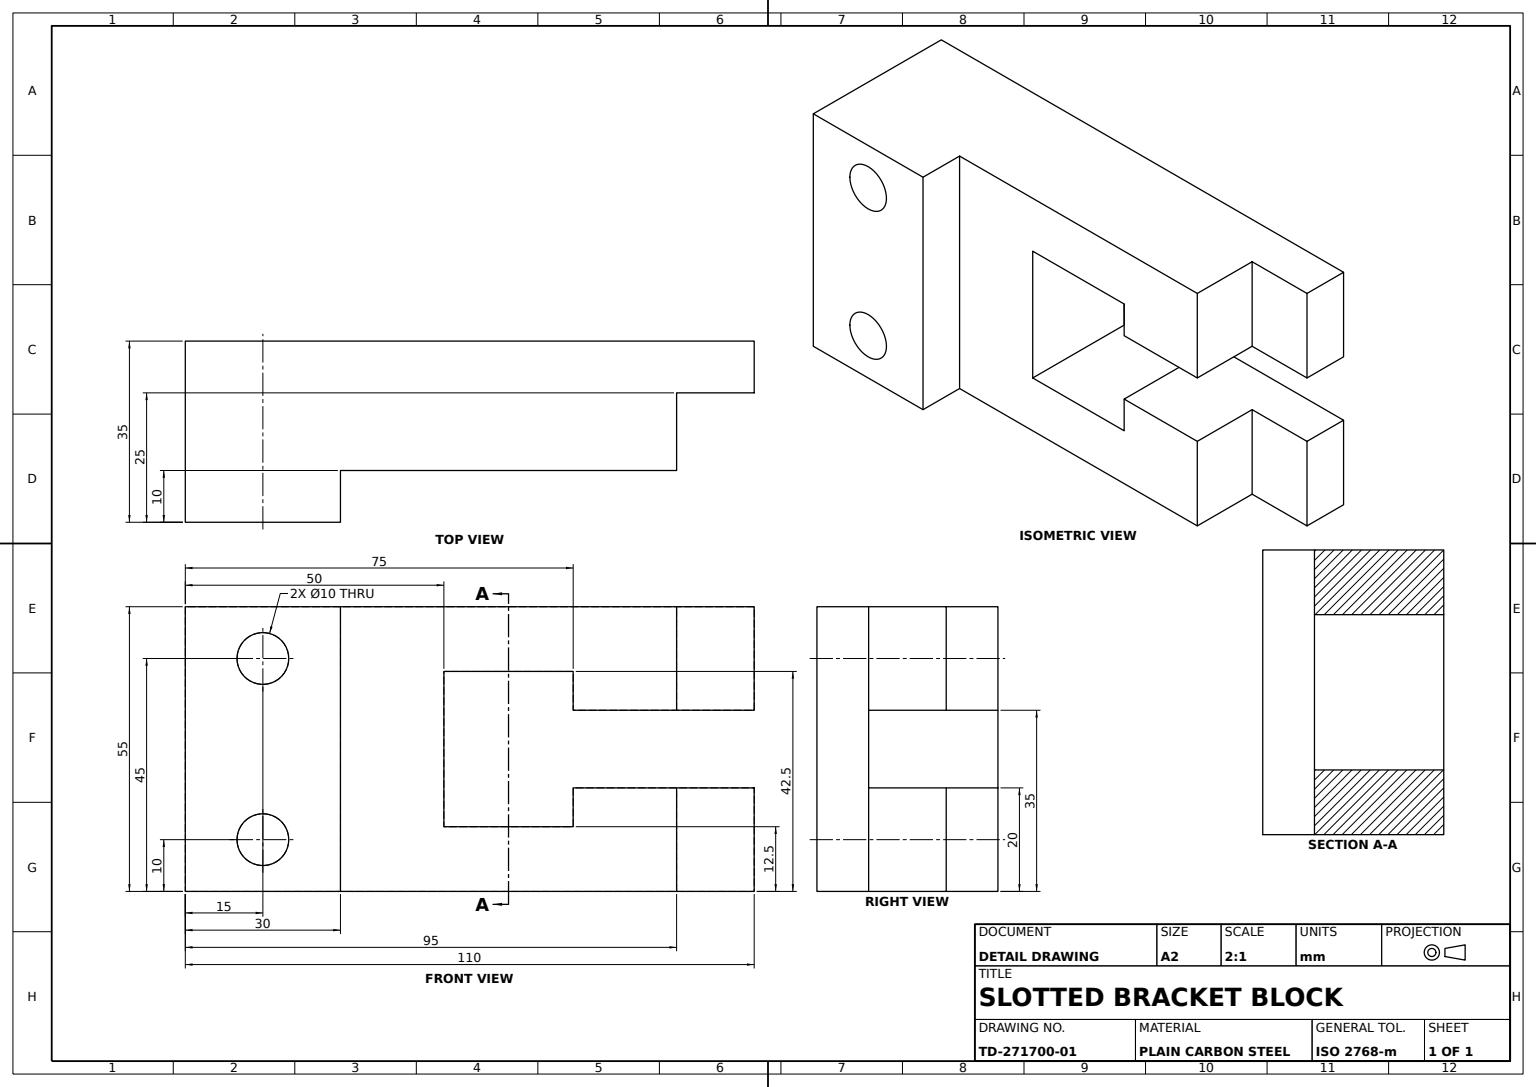
SolidWorks part; units mm, degrees
material "Plain Carbon Steel"
ref_plane "Front Plane" through (0, 0, 0) normal (0, 0, 1) x (1, 0, 0)
ref_plane "Top Plane" through (0, 0, 0) normal (0, 1, 0) x (1, 0, 0)
ref_plane "Right Plane" through (0, 0, 0) normal (1, 0, 0) x (0, 0, -1)
sketch "Base Profile Sketch" plane through (0, 0, 0) normal (0, 0, 1) x (1, 0, 0)
  line L0 (0, 0) -> (0, -55)
  line L1 (0, -55) -> (110, -55)
  line L2 (110, -55) -> (110, -35)
  line L3 (110, -35) -> (75, -35)
  line L4 (75, -35) -> (75, -42.5)
  line L5 (75, -42.5) -> (50, -42.5)
  line L6 (50, -42.5) -> (50, -12.5)
  line L7 (50, -12.5) -> (75, -12.5)
  line L8 (75, -12.5) -> (75, -20)
  line L9 (75, -20) -> (110, -20)
  line L10 (110, -20) -> (110, 0)
  line L11 (110, 0) -> (0, 0)
  dimension "D1" = 50
  dimension "D2" = 75
  dimension "D3" = 110
  dimension "D4" = 12.5
  dimension "D5" = 20
  dimension "D6" = 35
extrude "Base Profile" add sketch "Base Profile Sketch" along normal blind 10
sketch "Upright Block Sketch" plane through (0, 0, 10) normal (0, 0, 1) x (1, 0, 0)
  line L0 (0, -55) -> (110, -55) construction
  line L1 (0, 0) -> (30, 0)
  line L2 (0, 0) -> (0, -55)
  line L3 (0, -55) -> (30, -55)
  line L4 (30, 0) -> (30, -55)
  dimension "D1" = 30
extrude "Upright Block" add sketch "Upright Block Sketch" along normal blind 25
sketch "Slotted Arm Sketch" plane through (0, 0, 10) normal (0, 0, 1) x (1, 0, 0)
  line L0 (30, 0) -> (30, -55)
  line L1 (30, -55) -> (95, -55)
  line L2 (30, -55) -> (110, -55) construction
  line L3 (95, -55) -> (95, -35)
  line L4 (110, -35) -> (75, -35) construction
  line L5 (95, -35) -> (75, -35)
  line L6 (75, -35) -> (75, -42.5)
  line L7 (75, -42.5) -> (50, -42.5)
  line L8 (50, -42.5) -> (50, -12.5)
  line L9 (50, -12.5) -> (75, -12.5)
  line L10 (75, -12.5) -> (75, -20)
  line L11 (75, -20) -> (95, -20)
  line L12 (75, -20) -> (110, -20) construction
  line L13 (95, -20) -> (95, 0)
  line L14 (110, 0) -> (30, 0) construction
  line L15 (95, 0) -> (30, 0)
  line L16 (30, -55) -> (30, 0) construction
  dimension "D1" = 65
extrude "Slotted Arm" add sketch "Slotted Arm Sketch" along normal blind 15
sketch "Through Holes Sketch" plane through (0, 0, 35) normal (0, 0, 1) x (1, 0, 0)
  line L0 (30, 0) -> (0, 0) construction
  line L2 (0, 0) -> (0, -55) construction
  line L3 (0, -55) -> (30, -55) construction
  circle A0 centre (15, -10) radius 5
  circle A1 centre (15, -45) radius 5
  dimension "D1" = 10
  dimension "D2" = 10
  dimension "D8" = 10
  dimension "D3" = 10
  dimension "D4" = 10
  dimension "D5" = 15
  dimension "D6" = 15
  dimension "D7" = 35
extrude "Through Holes 2x" cut sketch "Through Holes Sketch" against normal blind 55
